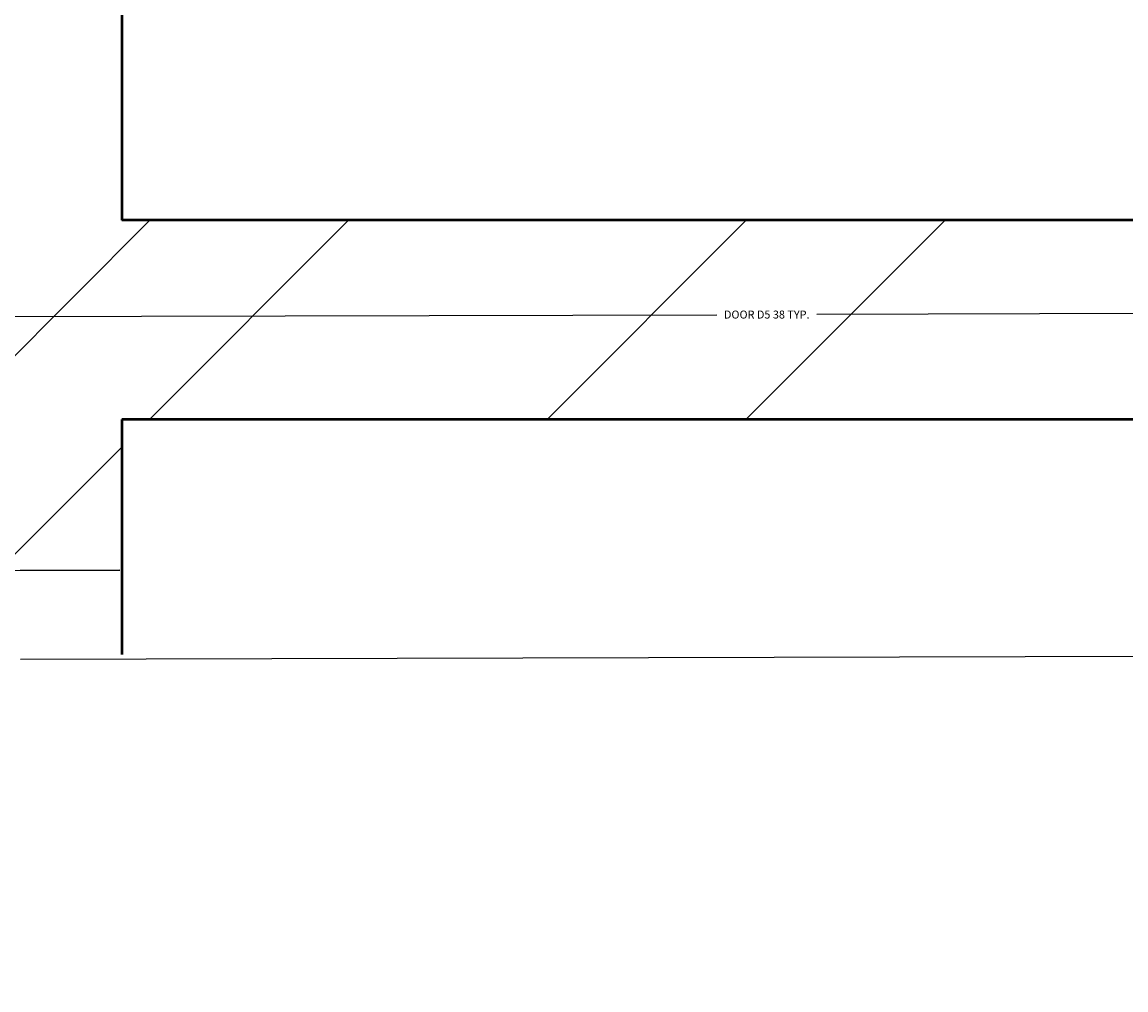
# Model space of a CAD drawing. Units: inches. Extents: x 963 to 2075, y 289 to 2657.
# Tile 9 of 98: x 1374 to 1399, y 1696 to 1718. Entities that reach past the tile are written whole.
import ezdxf

# ---------------------------------------------------------------- set-up
doc = ezdxf.new("R2010")
doc.units = ezdxf.units.IN
for name, color, linetype, lineweight in [('A-ANNO-DIMS', 2, 'Continuous', 18), ('A-DOOR', 4, 'Continuous', 25), ('A-WALL', 7, 'Continuous', 50), ('A-WALL-PATT', 8, 'Continuous', 13)]:
    doc.layers.add(name, color=color, linetype=linetype, lineweight=lineweight)
doc.styles.get("Standard").update_dxf_attribs({"font": 'arial.ttf'})
doc.dimstyles.get("Standard").update_dxf_attribs({"dimtxt": 0.18, "dimasz": 0.18, "dimexe": 0.18, "dimexo": 0.0625, "dimgap": 0.09, "dimtad": 0, "dimtih": 1, "dimtoh": 1, "dimdec": 4, "dimzin": 0, "dimdsep": 46, "dimtxsty": 'Standard', "dimcen": 0.09, "dimadec": 0, "dimazin": 0, "dimtfac": 1, "dimtdec": 4, "dimtofl": 0, "dimtmove": 0, "dimatfit": 3, "dimfxl": 1, "dimtolj": 1, "dimtzin": 0, "dimarcsym": 0})

# ---------------------------------------------------------------- blocks, each defined once
blk = doc.blocks.new('DOOR-5')
for p, q in [((29.907, 38.25), (29.907, 33.75)), ((27.907, 36), (27.907, 0)), ((29.907, 33.75), (29.907, 36))]:
    blk.add_line(p, q)
blk.add_arc((27.907, 27.321), 27.321, 161.4794, 270)
blk = doc.blocks.new('*D38')
at = {"layer": 'A-ANNO-DIMS', "color": 0, "lineweight": -2, "transparency": 16777216}
for p, q in [((1410.131, 1706.06), (1410.117, 1711.915)), ((1371.881, 1705.966), (1371.867, 1711.821)), ((1372.047, 1711.641), (1389.861, 1711.685)), ((1409.937, 1711.735), (1392.123, 1711.691))]:
    blk.add_line(p, q, dxfattribs=at)
at = {"layer": 'A-ANNO-DIMS', "color": 0, "transparency": 16777216}
for points in [[(1372.047, 1711.671), (1372.047, 1711.611), (1371.867, 1711.641)], [(1409.937, 1711.765), (1409.937, 1711.705), (1410.117, 1711.735)]]:
    blk.add_solid(points, dxfattribs=at)
at = {"layer": 'Defpoints', "color": 0, "transparency": 16777216}
for p in [(1371.867, 1711.641), (1410.131, 1705.998), (1371.881, 1705.903)]:
    blk.add_point(p, dxfattribs=at)
at = {"layer": 'A-ANNO-DIMS', "color": 0, "transparency": 16777216, "insert": (1390.992, 1711.688), "char_height": 0.18, "attachment_point": 5}
blk.add_mtext('\\A1;DOOR D5 38 TYP.', dxfattribs=at)

msp = doc.modelspace()

# ---------------------------------------------------------------- hatches: boundary and pattern name
at = {"layer": 'A-WALL-PATT'}
h = msp.add_hatch(dxfattribs=at)
h.set_pattern_fill('ANSI32', color=256)
h.paths.add_polyline_path([(1473.609, 2163.068), (1473.609, 2165.318), (1376.422, 2165.318), (1376.422, 2227.983), (1371.922, 2227.983), (1371.922, 2214.818), (1368.405, 2214.818), (1368.405, 2210.318), (1371.922, 2210.318), (1371.922, 2160.818), (1395.922, 2160.818), (1395.922, 2090.318), (1217.345, 2090.318), (1217.345, 2085.818), (1395.922, 2085.818), (1458.922, 2085.818), (1458.922, 2108.318), (1454.422, 2108.318), (1454.422, 2090.318), (1400.422, 2090.318), (1400.422, 2160.818), (1473.609, 2160.818)])
h.paths.add_polyline_path([(1649.422, 2210.318), (1653.225, 2210.318), (1653.225, 2214.818), (1649.422, 2214.818), (1649.422, 2227.983), (1644.922, 2227.983), (1644.922, 2165.318), (1550.099, 2165.318), (1550.099, 2160.818), (1620.922, 2160.818), (1620.922, 2112.818), (1555.446, 2112.818), (1555.446, 2108.318), (1584.327, 2108.318), (1584.327, 2084.916), (1588.827, 2084.916), (1588.827, 2108.318), (1625.422, 2108.318), (1667.951, 2108.318), (1667.951, 2022.667), (1588.827, 2022.667), (1588.827, 2047.408), (1584.327, 2047.408), (1584.327, 1996.003), (1588.827, 1996.003), (1588.827, 2018.318), (1667.951, 2018.167), (1667.951, 1928.318), (1625.422, 1928.318), (1625.422, 1923.818), (1672.451, 1923.818), (1672.451, 1928.318), (1672.451, 1946.663), (1785.446, 1946.663), (1785.446, 1951.163), (1743.034, 1951.163), (1743.034, 2017.922), (1841.422, 2017.922), (1841.422, 2014.775), (1845.922, 2014.775), (1845.922, 2017.922), (1905.922, 2017.922), (1905.922, 1987.511), (1910.422, 1987.511), (1910.422, 2022.422), (1910.422, 2068.517), (1905.922, 2068.517), (1905.922, 2022.422), (1845.922, 2022.422), (1845.922, 2025.851), (1843.672, 2025.851), (1841.422, 2025.851), (1841.422, 2022.422), (1743.034, 2022.422), (1743.034, 2084.031), (1768.451, 2084.031), (1785.446, 2084.031), (1785.446, 2088.531), (1672.451, 2088.531), (1672.451, 2112.818), (1667.951, 2112.818), (1625.422, 2112.818), (1625.422, 2160.818), (1649.422, 2160.818)])
h.paths.add_polyline_path([(1672.451, 2084.031), (1738.534, 2084.031), (1738.534, 1951.163), (1672.451, 1951.163)], flags=16)
h.paths.add_polyline_path([(1672.451, 2084.031), (1738.534, 2084.031), (1705.492, 2017.597)], flags=0)
h.paths.add_polyline_path([(1262.766, 2085.818), (1258.266, 2085.818), (1258.266, 2023.278), (1184.422, 2023.278), (1184.422, 2018.778), (1258.266, 2018.778), (1258.266, 1950.818), (1262.766, 1950.818)])
h.paths.add_polyline_path([(1312.266, 2085.818), (1307.766, 2085.818), (1307.766, 1950.818), (1312.266, 1950.818)])
h.paths.add_polyline_path([(1458.922, 1950.818), (1395.922, 1950.818), (1216.568, 1950.818), (1216.568, 1946.318), (1346.422, 1946.318), (1395.922, 1946.318), (1395.922, 1875.818), (1371.922, 1875.818), (1371.922, 1826.318), (1368.931, 1826.318), (1368.931, 1821.818), (1371.922, 1821.818), (1371.922, 1813.622), (1376.422, 1813.622), (1376.422, 1871.318), (1474.504, 1871.318), (1474.504, 1873.568), (1474.504, 1875.818), (1400.422, 1875.818), (1400.422, 1946.318), (1454.422, 1946.318), (1454.422, 1928.318), (1458.922, 1928.318)])
h.paths.add_polyline_path([(1184.422, 2120.778), (1167.922, 2120.778), (1167.922, 2134.812), (1165.672, 2134.812), (1163.422, 2134.812), (1163.422, 2120.778), (1119.922, 2120.778), (1119.922, 2098.095), (1124.422, 2098.095), (1124.422, 2116.278), (1167.922, 2116.278), (1179.922, 2116.278), (1179.922, 2045.916), (1184.422, 2045.916), (1184.422, 2090.318), (1184.422, 2116.278)])
h.paths.add_polyline_path([(1124.422, 2018.778), (1179.922, 2018.778), (1179.922, 2016.294), (1184.422, 2016.294), (1184.422, 2023.278), (1184.422, 2026.588), (1182.172, 2026.588), (1179.922, 2026.588), (1179.922, 2023.278), (1124.422, 2023.278), (1124.422, 2074.095), (1119.922, 2074.095), (1119.922, 2018.778), (1119.922, 1979.633), (1124.422, 1979.633)])
h.paths.add_polyline_path([(1184.422, 1925.778), (1184.422, 1946.318), (1184.422, 1996.073), (1182.172, 1996.073), (1179.922, 1996.073), (1179.922, 1925.778), (1124.422, 1925.778), (1124.422, 1955.633), (1119.922, 1955.502), (1119.922, 1921.278), (1158.922, 1921.278), (1158.922, 1909.983), (1163.422, 1909.983), (1163.422, 1921.278), (1184.422, 1921.278)])
h.paths.add_polyline_path([(1341.449, 1826.318), (1163.422, 1826.318), (1163.422, 1849.983), (1158.922, 1849.983), (1158.922, 1821.818), (1158.922, 1804.033), (1163.422, 1804.033), (1163.422, 1821.818), (1341.449, 1821.818)])
h.paths.add_polyline_path([(1222.981, 1713.818), (1163.422, 1713.818), (1163.422, 1744.033), (1161.172, 1744.033), (1158.922, 1744.033), (1158.922, 1713.818), (1119.922, 1713.818), (1119.922, 1694.65), (1124.422, 1694.65), (1124.422, 1709.318), (1158.922, 1709.318), (1222.981, 1709.318)])
h.paths.add_polyline_path([(1328.422, 1713.818), (1252.042, 1713.818), (1252.042, 1711.568), (1252.042, 1709.318), (1256.422, 1709.318), (1256.422, 1547.318), (1232.937, 1547.318), (1232.937, 1545.068), (1232.937, 1542.818), (1292.422, 1542.818), (1292.422, 1527.634), (1296.922, 1527.634), (1296.922, 1542.818), (1299.464, 1542.818), (1299.464, 1547.318), (1260.922, 1547.318), (1260.922, 1658.318), (1343.661, 1658.318), (1343.661, 1660.568), (1343.661, 1662.818), (1328.422, 1662.818), (1328.422, 1676.589), (1327.402, 1676.589), (1323.922, 1676.589), (1323.922, 1662.818), (1260.922, 1662.818), (1260.922, 1709.318), (1323.922, 1709.318), (1323.922, 1699.851), (1328.422, 1699.851)])
h.paths.add_polyline_path([(1649.422, 1875.818), (1625.422, 1875.818), (1625.422, 1928.318), (1620.922, 1928.318), (1588.827, 1928.318), (1588.827, 1950.59), (1584.327, 1950.59), (1584.327, 1928.318), (1555.446, 1928.318), (1555.446, 1923.818), (1620.922, 1923.818), (1620.922, 1875.818), (1548.952, 1875.818), (1548.952, 1873.568), (1548.952, 1871.318), (1644.922, 1871.318), (1644.922, 1813.622), (1649.422, 1813.622), (1649.422, 1821.818), (1652.045, 1821.818), (1652.045, 1824.068), (1652.045, 1826.318), (1649.422, 1826.318)])
h.paths.add_polyline_path([(1512.922, 1871.318), (1516.476, 1871.318), (1516.476, 1875.818), (1512.922, 1875.818), (1512.922, 1923.818), (1512.922, 1928.318), (1512.922, 1930.827), (1508.422, 1930.827), (1508.422, 1875.818), (1504.411, 1875.818), (1504.411, 1871.318), (1508.422, 1871.318), (1508.422, 1713.818), (1376.422, 1713.818), (1376.422, 1743.325), (1371.922, 1743.325), (1371.922, 1709.318), (1371.922, 1706.01), (1376.422, 1706.01), (1376.422, 1709.318), (1508.422, 1709.318), (1508.422, 1547.318), (1501.871, 1547.318), (1501.871, 1542.818), (1508.422, 1542.818), (1508.422, 1482.818), (1508.422, 1436.318), (1512.922, 1436.318), (1512.922, 1542.818), (1519.318, 1542.818), (1519.318, 1545.068), (1519.318, 1547.318), (1512.922, 1547.318), (1512.922, 1709.318), (1644.922, 1709.318), (1644.922, 1707.548), (1649.422, 1707.548), (1649.422, 1709.318), (1649.422, 1743.325), (1644.922, 1743.325), (1644.922, 1713.818), (1512.922, 1713.818)])
h.paths.add_polyline_path([(1129.884, 1545.068), (1129.884, 1547.318), (1124.422, 1547.318), (1095.922, 1547.318), (1095.922, 1614.818), (1124.422, 1614.818), (1124.422, 1619.318), (1095.922, 1619.318), (1091.422, 1619.318), (1091.422, 1542.818), (1095.922, 1542.818), (1119.922, 1542.818), (1129.884, 1542.818)])
h.paths.add_polyline_path([(1208.422, 1542.818), (1211.74, 1542.818), (1211.74, 1547.318), (1198.851, 1547.318), (1198.851, 1542.818), (1203.922, 1542.818), (1203.922, 1478.318), (1208.422, 1478.318), (1296.922, 1478.318), (1296.922, 1503.634), (1292.422, 1503.634), (1292.422, 1482.818), (1208.422, 1482.818)])
h.paths.add_polyline_path([(1430.422, 1542.818), (1435.699, 1542.818), (1435.699, 1545.068), (1435.699, 1547.318), (1422.658, 1547.318), (1422.658, 1545.068), (1422.658, 1542.818), (1425.922, 1542.818), (1425.922, 1482.857), (1341.922, 1482.857), (1341.922, 1502.732), (1337.422, 1502.732), (1337.422, 1478.357), (1425.922, 1478.357), (1425.922, 1440.818), (1425.922, 1436.318), (1430.422, 1436.318)])
h.paths.add_polyline_path([(1698.482, 2004.259), (1727.695, 2004.259), (1727.695, 2022.916), (1698.482, 2022.916)], flags=8)

# ---------------------------------------------------------------- linework, layer by layer
at = {"layer": 'A-WALL'}
for p, q in [((1376.422, 1743.325), (1376.422, 1713.818)), ((1508.422, 1713.818), (1376.422, 1713.818)), ((1508.422, 1709.318), (1376.422, 1709.318)), ((1376.422, 1709.318), (1376.422, 1704.01))]:
    msp.add_line(p, q, dxfattribs=at)

# ---------------------------------------------------------------- block references
at = {"layer": 'A-DOOR', "rotation": 90.14142652708767}
msp.add_blockref('DOOR-5', (1410.204, 1676.091), dxfattribs=at)

# ---------------------------------------------------------------- dimensions: what is measured, and where the dimension line sits
at = {"layer": 'A-ANNO-DIMS'}
dim = msp.add_linear_dim(base=(1371.867, 1711.641), p1=(1410.131, 1705.998), p2=(1371.881, 1705.903), angle=180.1414, text='DOOR D5 <> TYP.', dimstyle='Standard', override={"dimdec": 0, "dimlfac": 1, "dimrnd": 0, "dimzin": 0, "dimdsep": 46, "dimlunit": 2}, dxfattribs=at)
dim.commit()
dim.dimension.update_dxf_attribs({"geometry": '*D38', "text_midpoint": (1390.992, 1711.688)})

doc.saveas('drawing.dxf')
